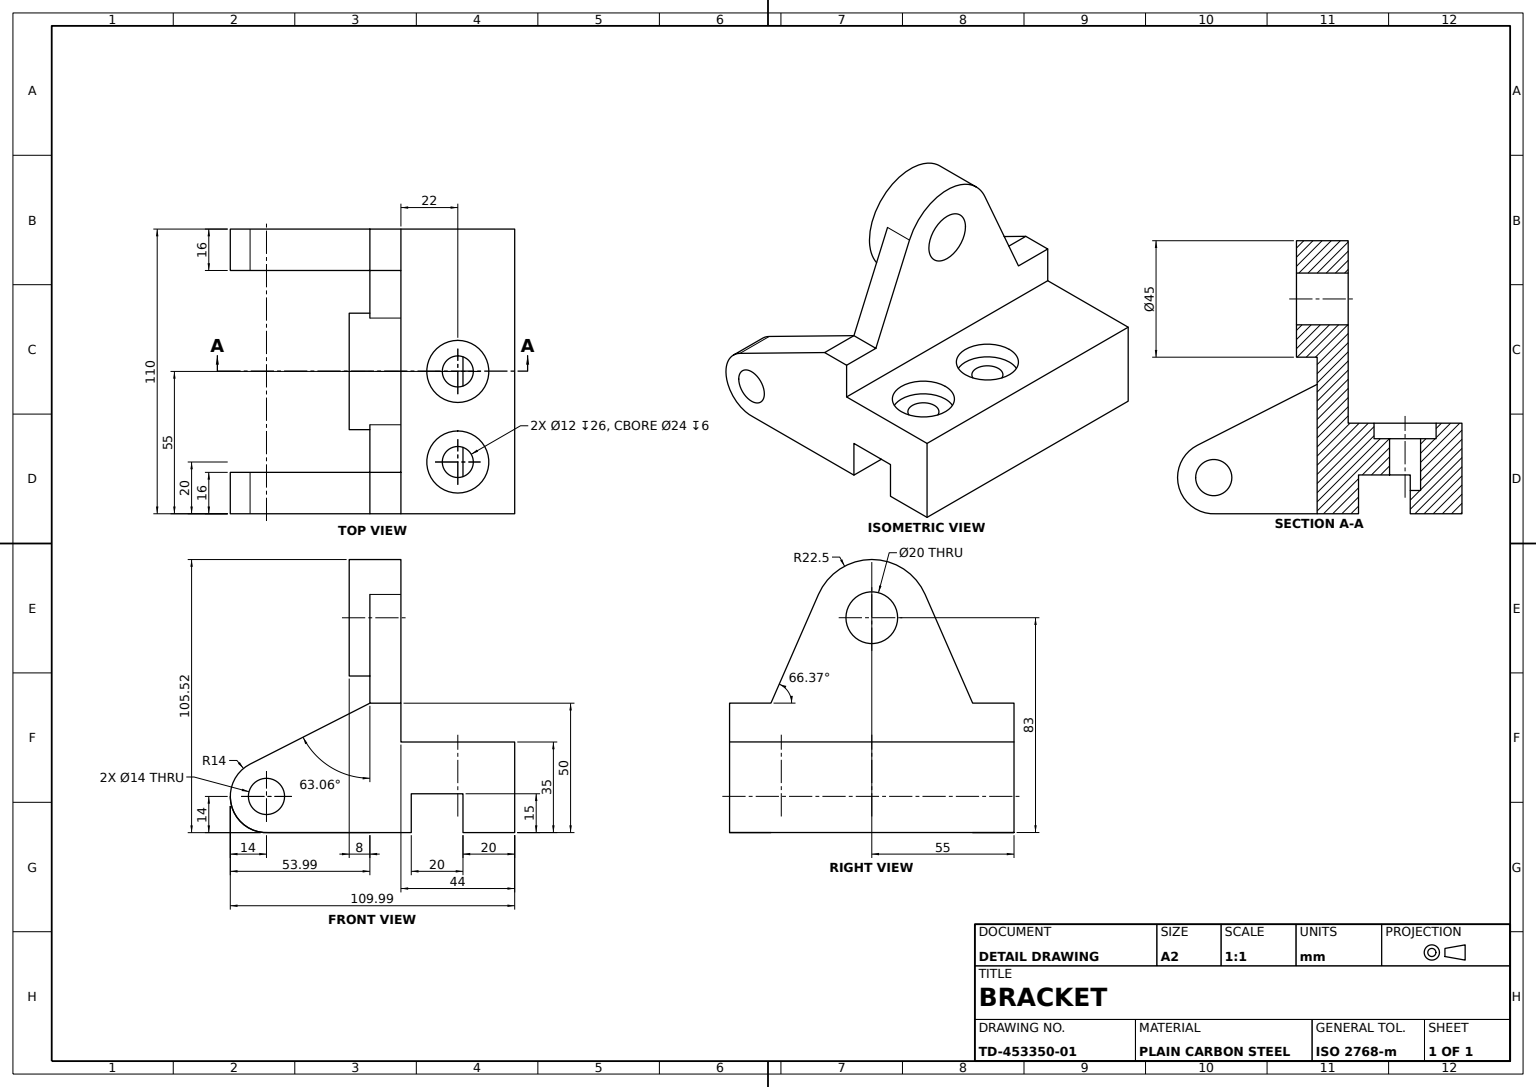
from build123d import *

# Parameters (mm, degrees)
BASE_BLOCK_SKETCH_W         = 56
BASE_BLOCK_SKETCH_H         = 35
BASE_BLOCK_DEPTH            = 110
BOTTOM_SLOT_SKETCH_W        = 20
BOTTOM_SLOT_SKETCH_H        = 15
BOTTOM_SLOT_DEPTH           = 110
SIDE_STEP_SKETCH_W          = 12
SIDE_STEP_SKETCH_H          = 15
SIDE_STEP_DEPTH             = 110
SIDE_LUG_1_DEPTH            = 16
SIDE_HOLE_1_SKETCH_R        = 7
SIDE_HOLE_1_DEPTH           = 16
SIDE_START                  = -16
SIDE_LUG_2_DEPTH            = 16
SIDE_HOLE_2_SKETCH_R        = 7
SIDE_HOLE_2_DEPTH           = 16
UPRIGHT_EAR_DEPTH           = 12
PIVOT_START                 = 8
PIVOT_BOSS_45_SKETCH_R      = 22.5
PIVOT_BOSS_45_DEPTH         = 8
PIVOT_BORE_20_SKETCH_R      = 10
PIVOT_BORE_20_DEPTH         = 20
COUNTERBORES_2X_24_SKETCH_R = 12
COUNTERBORES_2X_24_DEPTH    = 6
HOLES_2X_12_SKETCH_R        = 6
HOLES_2X_12_DEPTH           = 20


with BuildPart() as part:
    # Base Block Sketch → Base Block (new body)
    with BuildSketch(Plane.XY):
        with Locations((22, 17.5)):
            Rectangle(BASE_BLOCK_SKETCH_W, BASE_BLOCK_SKETCH_H)
    extrude(amount=BASE_BLOCK_DEPTH)

    # Bottom Slot Sketch → Bottom Slot (cut)
    with BuildSketch(Plane.XY.offset(110)):
        with Locations((20, 7.5)):
            Rectangle(BOTTOM_SLOT_SKETCH_W, BOTTOM_SLOT_SKETCH_H)
    extrude(amount=-BOTTOM_SLOT_DEPTH, mode=Mode.SUBTRACT)

    # Side Step Sketch → Side Step (add)
    with BuildSketch(Plane.XY.offset(110)):
        with Locations((0, 42.5)):
            Rectangle(SIDE_STEP_SKETCH_W, SIDE_STEP_SKETCH_H)
    extrude(amount=-SIDE_STEP_DEPTH)

    # Side Lug 1 Sketch → Side Lug 1 (add)
    with BuildSketch(Plane.XY.offset(110)):
        with BuildLine():
            Line((-45.151057186, 0), (-6, 0))
            Line((-6, 0), (-6, 50))
            Line((-6, 50), (-52.329877609, 26.455854883))
            ThreePointArc((-52.329877609, 26.455854883), (-59.498699864, 10.308671221), (-45.151057186, 0))
        make_face()
    extrude(amount=-SIDE_LUG_1_DEPTH)

    # Side Hole 1 Sketch → Side Hole 1 (cut)
    with BuildSketch(Plane.XY.offset(110)):
        with Locations((-45.987296801, 13.975002802)):
            Circle(SIDE_HOLE_1_SKETCH_R)
    extrude(amount=-SIDE_HOLE_1_DEPTH, mode=Mode.SUBTRACT)

    # Side Lug 2 Sketch → Side Lug 2 (add)
    with BuildSketch(Plane(origin=(0, 0, 0), x_dir=(-1, 0, 0), z_dir=(0, 0, -1)).offset(SIDE_START)):
        with BuildLine():
            Line((6, 50), (6, 0))
            Line((6, 0), (45.151057186, 0))
            ThreePointArc((45.151057186, 0), (59.498699864, 10.308671221), (52.329877609, 26.455854883))
            Line((52.329877609, 26.455854883), (6, 50))
        make_face()
    extrude(amount=SIDE_LUG_2_DEPTH)

    # Side Hole 2 Sketch → Side Hole 2 (cut)
    with BuildSketch(Plane(origin=(0, 0, 0), x_dir=(-1, 0, 0), z_dir=(0, 0, -1)).offset(SIDE_START)):
        with Locations(Location((45.987296801, 13.975002802, 0), (0, 0, 180))):
            Circle(SIDE_HOLE_2_SKETCH_R)
    extrude(amount=SIDE_HOLE_2_DEPTH, mode=Mode.SUBTRACT)

    # Upright Ear Sketch → Upright Ear (add)
    with BuildSketch(Plane.ZY.offset(6)):
        with BuildLine():
            Line((34.387072411, 92.019823514), (16, 50))
            Line((16, 50), (94, 50))
            Line((94, 50), (75.612927589, 92.019823514))
            ThreePointArc((75.612927589, 92.019823514), (55, 105.5), (34.387072411, 92.019823514))
        make_face()
    extrude(amount=-UPRIGHT_EAR_DEPTH)

    # Pivot Boss Ø45 Sketch → Pivot Boss Ø45 (add)
    with BuildSketch(Plane.ZY.offset(6).offset(PIVOT_START)):
        with Locations((55, 83)):
            Circle(PIVOT_BOSS_45_SKETCH_R)
    extrude(amount=-PIVOT_BOSS_45_DEPTH)

    # Pivot Bore Ø20 Sketch → Pivot Bore Ø20 (cut)
    with BuildSketch(Plane.ZY.offset(14)):
        with Locations((55, 83)):
            Circle(PIVOT_BORE_20_SKETCH_R)
    extrude(amount=-PIVOT_BORE_20_DEPTH, mode=Mode.SUBTRACT)

    # Counterbores 2xØ24 Sketch → Counterbores 2xØ24 (cut)
    with BuildSketch(Plane(origin=(0, 35, 0), x_dir=(1, 0, 0), z_dir=(0, 1, 0))):
        with Locations(Location((28, -90, 0), (0, 0, 270))):
            Circle(COUNTERBORES_2X_24_SKETCH_R)
        with Locations(Location((28, -55, 0), (0, 0, 270))):
            Circle(COUNTERBORES_2X_24_SKETCH_R)
    extrude(amount=-COUNTERBORES_2X_24_DEPTH, mode=Mode.SUBTRACT)

    # Holes 2xØ12 Sketch → Holes 2xØ12 (cut)
    with BuildSketch(Plane(origin=(0, 29, 0), x_dir=(1, 0, 0), z_dir=(0, 1, 0))):
        with Locations(Location((28, -55, 0), (0, 0, 270))):
            Circle(HOLES_2X_12_SKETCH_R)
        with Locations(Location((28, -90, 0), (0, 0, 270))):
            Circle(HOLES_2X_12_SKETCH_R)
    extrude(amount=-HOLES_2X_12_DEPTH, mode=Mode.SUBTRACT)


solid = part.part
